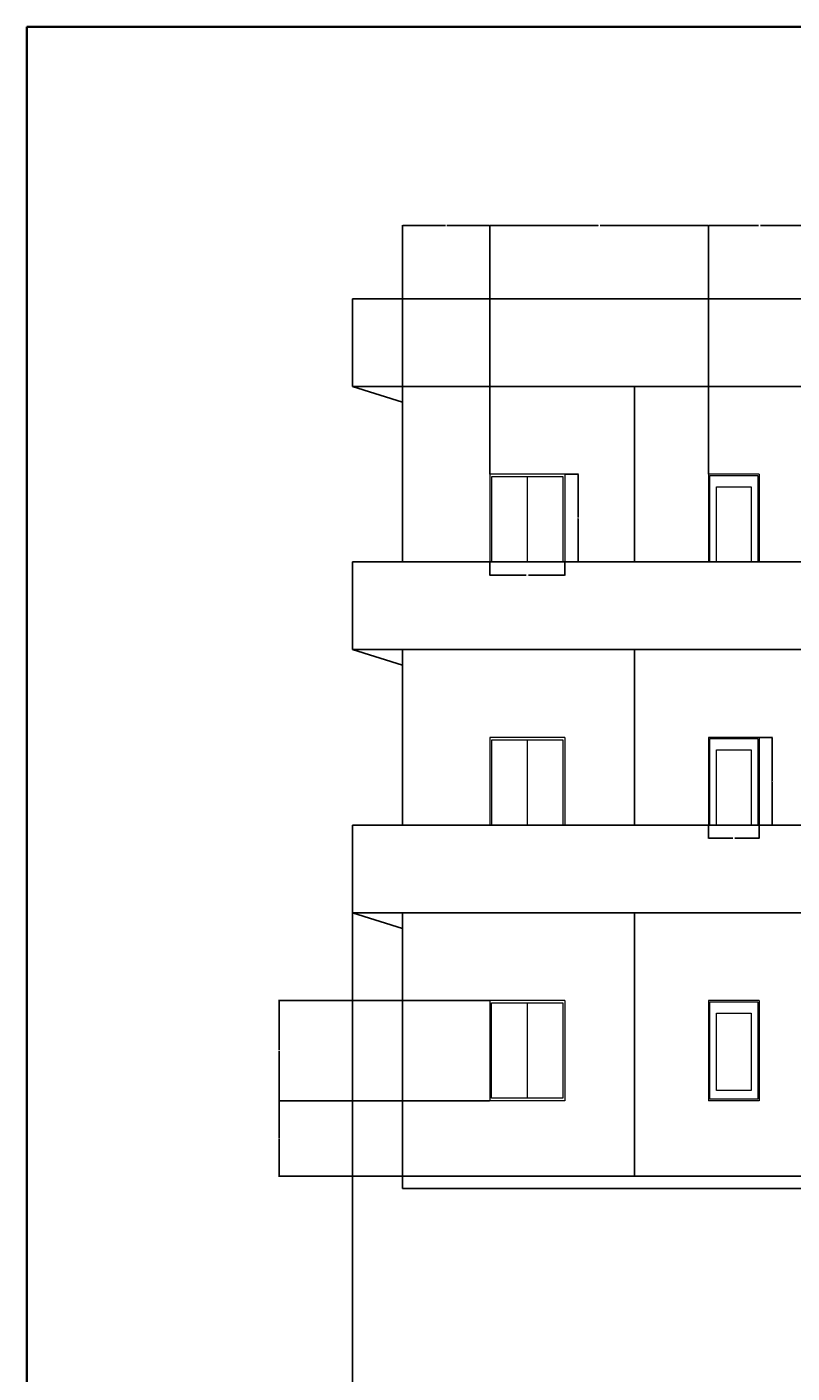
# Model space of a CAD drawing. Units: inches. Extents: x 1520 to 3401, y 1570 to 3432.
# Tile 8 of 15: x 1520 to 1886, y 2787 to 3432. Entities that reach past the tile are written whole.
import ezdxf

# ---------------------------------------------------------------- set-up
doc = ezdxf.new("R2010")
doc.units = ezdxf.units.IN
for name, color, linetype, lineweight in [('A-ANNO-DIMS', 2, 'Continuous', 18), ('A-ANNO-TTLB', 7, 'Continuous', 35), ('A-ELEV', 7, 'Continuous', 25), ('A-ELEV-GLAZ', 4, 'Continuous', 18)]:
    doc.layers.add(name, color=color, linetype=linetype, lineweight=lineweight)
doc.styles.get("Standard").update_dxf_attribs({"font": 'arial.ttf'})
doc.dimstyles.get("Standard").update_dxf_attribs({"dimtxt": 0.18, "dimasz": 0.18, "dimexe": 0.18, "dimexo": 0.0625, "dimgap": 0.09, "dimtad": 0, "dimtih": 1, "dimtoh": 1, "dimdec": 4, "dimzin": 0, "dimdsep": 46, "dimtxsty": 'Standard', "dimcen": 0.09, "dimadec": 0, "dimazin": 0, "dimtfac": 1, "dimtdec": 4, "dimtofl": 0, "dimtmove": 0, "dimatfit": 3, "dimfxl": 1, "dimtolj": 1, "dimtzin": 0, "dimarcsym": 0})

# ---------------------------------------------------------------- blocks, each defined once
blk = doc.blocks.new('WIN-ELEV-01')
for p, q in [((0, 42), (0, 0)), ((36, 42), (0, 42)), ((0, 42), (0, 0)), ((36, 42), (0, 42)), ((17.97, 40.89), (17.97, 0)), ((36, 42), (36, 0)), ((36, 42), (36, 0))]:
    blk.add_line(p, q)
blk.add_lwpolyline([(0.93, 0), (0.93, 40.89), (35, 40.89), (35, 0)])
blk = doc.blocks.new('WIN-ELEV-02')
for p, q in [((0, 42), (0, 0)), ((24.17, 42), (0, 42)), ((0, 42), (0, 0)), ((24.17, 42), (0, 42)), ((24.17, 42), (24.17, 0)), ((24.17, 42), (24.17, 0))]:
    blk.add_line(p, q)
for points in [[(0.65, 0), (0.65, 41.38), (23.63, 41.38), (23.63, 0)], [(3.78, 0), (3.78, 35.97), (20.43, 35.97), (20.43, 0)]]:
    blk.add_lwpolyline(points)
blk = doc.blocks.new('*D157')
at = {"layer": 'A-ANNO-DIMS', "color": 0, "lineweight": -2, "transparency": 16777216}
for p, q in [((1777.36, 3217.63), (1783.78, 3217.63)), ((1783.6, 3217.45), (1783.6, 3196.81)), ((1783.6, 3175.81), (1783.6, 3196.45)), ((1777.36, 3175.63), (1783.78, 3175.63))]:
    blk.add_line(p, q, dxfattribs=at)
at = {"layer": 'A-ANNO-DIMS', "color": 0, "transparency": 16777216}
for points in [[(1783.57, 3217.45), (1783.63, 3217.45), (1783.6, 3217.63)], [(1783.57, 3175.81), (1783.63, 3175.81), (1783.6, 3175.63)]]:
    blk.add_solid(points, dxfattribs=at)
at = {"layer": 'Defpoints', "color": 0, "transparency": 16777216}
for p in [(1777.3, 3217.63), (1783.6, 3217.63), (1777.3, 3175.63)]:
    blk.add_point(p, dxfattribs=at)
at = {"layer": 'A-ANNO-DIMS', "color": 0, "transparency": 16777216, "insert": (1783.6, 3196.63), "char_height": 0.18, "attachment_point": 5}
blk.add_mtext('\\A1;EW1 42 TYP.', dxfattribs=at)
blk = doc.blocks.new('*D158')
at = {"layer": 'A-ANNO-DIMS', "color": 0, "lineweight": -2, "transparency": 16777216}
for p, q in [((1741.3, 3175.57), (1741.3, 3169.15)), ((1777.3, 3175.57), (1777.3, 3169.15)), ((1741.48, 3169.33), (1758.77, 3169.33)), ((1777.12, 3169.33), (1759.82, 3169.33))]:
    blk.add_line(p, q, dxfattribs=at)
at = {"layer": 'A-ANNO-DIMS', "color": 0, "transparency": 16777216}
for points in [[(1741.48, 3169.36), (1741.48, 3169.3), (1741.3, 3169.33)], [(1777.12, 3169.36), (1777.12, 3169.3), (1777.3, 3169.33)]]:
    blk.add_solid(points, dxfattribs=at)
at = {"layer": 'Defpoints', "color": 0, "transparency": 16777216}
for p in [(1741.3, 3175.63), (1777.3, 3175.63), (1777.3, 3169.33)]:
    blk.add_point(p, dxfattribs=at)
at = {"layer": 'A-ANNO-DIMS', "color": 0, "transparency": 16777216, "insert": (1759.3, 3169.33), "char_height": 0.18, "attachment_point": 5}
blk.add_mtext('\\A1;36 TYP.', dxfattribs=at)
blk = doc.blocks.new('*D159')
at = {"layer": 'A-ANNO-DIMS', "color": 0, "lineweight": -2, "transparency": 16777216}
for p, q in [((1870.19, 3091.63), (1876.61, 3091.63)), ((1876.43, 3091.45), (1876.43, 3070.81)), ((1876.43, 3049.81), (1876.43, 3070.45)), ((1870.19, 3049.63), (1876.61, 3049.63))]:
    blk.add_line(p, q, dxfattribs=at)
at = {"layer": 'A-ANNO-DIMS', "color": 0, "transparency": 16777216}
for points in [[(1876.4, 3091.45), (1876.46, 3091.45), (1876.43, 3091.63)], [(1876.4, 3049.81), (1876.46, 3049.81), (1876.43, 3049.63)]]:
    blk.add_solid(points, dxfattribs=at)
at = {"layer": 'Defpoints', "color": 0, "transparency": 16777216}
for p in [(1870.13, 3091.63), (1876.43, 3091.63), (1870.13, 3049.63)]:
    blk.add_point(p, dxfattribs=at)
at = {"layer": 'A-ANNO-DIMS', "color": 0, "transparency": 16777216, "insert": (1876.43, 3070.63), "char_height": 0.18, "attachment_point": 5}
blk.add_mtext('\\A1;EW2 42 TYP.', dxfattribs=at)
blk = doc.blocks.new('*D160')
at = {"layer": 'A-ANNO-DIMS', "color": 0, "lineweight": -2, "transparency": 16777216}
for p, q in [((1845.96, 3049.57), (1845.96, 3043.15)), ((1870.13, 3049.57), (1870.13, 3043.15)), ((1846.14, 3043.33), (1857.51, 3043.33)), ((1869.95, 3043.33), (1858.57, 3043.33))]:
    blk.add_line(p, q, dxfattribs=at)
at = {"layer": 'A-ANNO-DIMS', "color": 0, "transparency": 16777216}
for points in [[(1846.14, 3043.36), (1846.14, 3043.3), (1845.96, 3043.33)], [(1869.95, 3043.36), (1869.95, 3043.3), (1870.13, 3043.33)]]:
    blk.add_solid(points, dxfattribs=at)
at = {"layer": 'Defpoints', "color": 0, "transparency": 16777216}
for p in [(1845.96, 3049.63), (1870.13, 3049.63), (1870.13, 3043.33)]:
    blk.add_point(p, dxfattribs=at)
at = {"layer": 'A-ANNO-DIMS', "color": 0, "transparency": 16777216, "insert": (1858.04, 3043.33), "char_height": 0.18, "attachment_point": 5}
blk.add_mtext('\\A1;24 TYP.', dxfattribs=at)
blk = doc.blocks.new('*D209')
at = {"layer": 'A-ANNO-DIMS', "color": 0, "lineweight": -2, "transparency": 16777216}
for p, q in [((1675.61, 3007.57), (1675.61, 2752.86)), ((2368.11, 3007.57), (2368.11, 2752.86)), ((1675.79, 2753.04), (2021.47, 2753.04)), ((2367.93, 2753.04), (2022.26, 2753.04))]:
    blk.add_line(p, q, dxfattribs=at)
at = {"layer": 'A-ANNO-DIMS', "color": 0, "transparency": 16777216}
for points in [[(1675.79, 2753.07), (1675.79, 2753.01), (1675.61, 2753.04)], [(2367.93, 2753.07), (2367.93, 2753.01), (2368.11, 2753.04)]]:
    blk.add_solid(points, dxfattribs=at)
at = {"layer": 'Defpoints', "color": 0, "transparency": 16777216}
for p in [(1675.61, 3007.63), (2368.11, 3007.63), (2368.11, 2753.04)]:
    blk.add_point(p, dxfattribs=at)
at = {"layer": 'A-ANNO-DIMS', "color": 0, "transparency": 16777216, "insert": (2021.86, 2753.04), "char_height": 0.18, "attachment_point": 5}
blk.add_mtext('\\A1;692.5', dxfattribs=at)
blk = doc.blocks.new('*D212')
at = {"layer": 'A-ANNO-DIMS', "color": 0, "lineweight": -2, "transparency": 16777216}
for p, q in [((1741.23, 2917.63), (1640.33, 2917.63)), ((1640.51, 2917.45), (1640.51, 2899.81)), ((1640.51, 2881.81), (1640.51, 2899.45)), ((1699.55, 2881.63), (1640.33, 2881.63))]:
    blk.add_line(p, q, dxfattribs=at)
at = {"layer": 'A-ANNO-DIMS', "color": 0, "transparency": 16777216}
for points in [[(1640.48, 2917.45), (1640.54, 2917.45), (1640.51, 2917.63)], [(1640.48, 2881.81), (1640.54, 2881.81), (1640.51, 2881.63)]]:
    blk.add_solid(points, dxfattribs=at)
at = {"layer": 'Defpoints', "color": 0, "transparency": 16777216}
for p in [(1640.51, 2917.63), (1741.3, 2917.63), (1699.61, 2881.63)]:
    blk.add_point(p, dxfattribs=at)
at = {"layer": 'A-ANNO-DIMS', "color": 0, "transparency": 16777216, "insert": (1640.51, 2899.63), "char_height": 0.18, "attachment_point": 5}
blk.add_mtext('\\A1;36', dxfattribs=at)
blk = doc.blocks.new('*D213')
at = {"layer": 'A-ANNO-DIMS', "color": 0, "lineweight": -2, "transparency": 16777216}
for p, q in [((1741.23, 2965.63), (1640.33, 2965.63)), ((1640.51, 2965.45), (1640.51, 2941.81)), ((1640.51, 2917.81), (1640.51, 2941.45)), ((1741.23, 2917.63), (1640.33, 2917.63))]:
    blk.add_line(p, q, dxfattribs=at)
at = {"layer": 'A-ANNO-DIMS', "color": 0, "transparency": 16777216}
for points in [[(1640.48, 2965.45), (1640.54, 2965.45), (1640.51, 2965.63)], [(1640.48, 2917.81), (1640.54, 2917.81), (1640.51, 2917.63)]]:
    blk.add_solid(points, dxfattribs=at)
at = {"layer": 'Defpoints', "color": 0, "transparency": 16777216}
for p in [(1640.51, 2965.63), (1741.3, 2965.63), (1741.3, 2917.63)]:
    blk.add_point(p, dxfattribs=at)
at = {"layer": 'A-ANNO-DIMS', "color": 0, "transparency": 16777216, "insert": (1640.51, 2941.63), "char_height": 0.18, "attachment_point": 5}
blk.add_mtext('\\A1;48', dxfattribs=at)
blk = doc.blocks.new('*D215')
at = {"layer": 'A-ANNO-DIMS', "color": 0, "lineweight": -2, "transparency": 16777216}
for p, q in [((1699.61, 3259.7), (1699.61, 3336.91)), ((1699.79, 3336.73), (1720.06, 3336.73)), ((1741.12, 3336.73), (1720.85, 3336.73)), ((1741.3, 3217.7), (1741.3, 3336.91))]:
    blk.add_line(p, q, dxfattribs=at)
at = {"layer": 'A-ANNO-DIMS', "color": 0, "transparency": 16777216}
for points in [[(1699.79, 3336.76), (1699.79, 3336.7), (1699.61, 3336.73)], [(1741.12, 3336.76), (1741.12, 3336.7), (1741.3, 3336.73)]]:
    blk.add_solid(points, dxfattribs=at)
at = {"layer": 'Defpoints', "color": 0, "transparency": 16777216}
for p in [(1741.3, 3336.73), (1699.61, 3259.63), (1741.3, 3217.63)]:
    blk.add_point(p, dxfattribs=at)
at = {"layer": 'A-ANNO-DIMS', "color": 0, "transparency": 16777216, "insert": (1720.45, 3336.73), "char_height": 0.18, "attachment_point": 5}
blk.add_mtext('\\A1;41.68', dxfattribs=at)
blk = doc.blocks.new('*D216')
at = {"layer": 'A-ANNO-DIMS', "color": 0, "lineweight": -2, "transparency": 16777216}
for p, q in [((1741.3, 3217.7), (1741.3, 3336.91)), ((1741.48, 3336.73), (1793.17, 3336.73)), ((1845.78, 3336.73), (1794.08, 3336.73)), ((1845.96, 3217.7), (1845.96, 3336.91))]:
    blk.add_line(p, q, dxfattribs=at)
at = {"layer": 'A-ANNO-DIMS', "color": 0, "transparency": 16777216}
for points in [[(1741.48, 3336.76), (1741.48, 3336.7), (1741.3, 3336.73)], [(1845.78, 3336.76), (1845.78, 3336.7), (1845.96, 3336.73)]]:
    blk.add_solid(points, dxfattribs=at)
at = {"layer": 'Defpoints', "color": 0, "transparency": 16777216}
for p in [(1845.96, 3336.73), (1741.3, 3217.63), (1845.96, 3217.63)]:
    blk.add_point(p, dxfattribs=at)
at = {"layer": 'A-ANNO-DIMS', "color": 0, "transparency": 16777216, "insert": (1793.63, 3336.73), "char_height": 0.18, "attachment_point": 5}
blk.add_mtext('\\A1;104.66', dxfattribs=at)
blk = doc.blocks.new('*D217')
at = {"layer": 'A-ANNO-DIMS', "color": 0, "lineweight": -2, "transparency": 16777216}
for p, q in [((1845.96, 3217.7), (1845.96, 3336.91)), ((1846.14, 3336.73), (1869.94, 3336.73)), ((1894.55, 3336.73), (1870.74, 3336.73)), ((1894.73, 3217.7), (1894.73, 3336.91))]:
    blk.add_line(p, q, dxfattribs=at)
at = {"layer": 'A-ANNO-DIMS', "color": 0, "transparency": 16777216}
for points in [[(1846.14, 3336.76), (1846.14, 3336.7), (1845.96, 3336.73)], [(1894.55, 3336.76), (1894.55, 3336.7), (1894.73, 3336.73)]]:
    blk.add_solid(points, dxfattribs=at)
at = {"layer": 'Defpoints', "color": 0, "transparency": 16777216}
for p in [(1894.73, 3336.73), (1845.96, 3217.63), (1894.73, 3217.63)]:
    blk.add_point(p, dxfattribs=at)
at = {"layer": 'A-ANNO-DIMS', "color": 0, "transparency": 16777216, "insert": (1870.34, 3336.73), "char_height": 0.18, "attachment_point": 5}
blk.add_mtext('\\A1;48.77', dxfattribs=at)

msp = doc.modelspace()

# ---------------------------------------------------------------- linework, layer by layer
at = {"layer": 'A-ANNO-TTLB'}
msp.add_lwpolyline([(1519.9253, 3431.7421), (3400.8761, 3431.7421), (3400.8761, 1570.3458), (1519.9253, 1570.3458)], close=True, dxfattribs=at)
at = {"layer": 'A-ELEV'}
for p, q in [((2368.1128, 3301.633), (1675.6128, 3301.633)), ((1675.6128, 3259.633), (1675.6128, 3301.633)), ((2368.1128, 3259.633), (1675.6128, 3259.633)), ((1675.6128, 3259.633), (1699.6128, 3252.133)), ((1699.6128, 3259.633), (1699.6128, 3175.633)), ((1810.5002, 3175.633), (1810.5002, 3259.633)), ((2368.1128, 3175.633), (1675.6128, 3175.633)), ((1675.6128, 3133.633), (1675.6128, 3175.633)), ((2368.1128, 3133.633), (1675.6128, 3133.633)), ((1675.6128, 3133.633), (1699.6128, 3126.133)), ((1699.6128, 3133.633), (1699.6128, 3049.633)), ((1699.6128, 3133.633), (1699.6128, 3118.633)), ((1810.5002, 3049.633), (1810.5002, 3133.633)), ((2368.1128, 3049.633), (1675.6128, 3049.633)), ((1675.6128, 3007.633), (1675.6128, 3049.633)), ((2368.1128, 3007.633), (1675.6128, 3007.633)), ((1675.6128, 3007.633), (1699.6128, 3000.133)), ((1699.6128, 3007.633), (1699.6128, 2875.633)), ((1699.6128, 3007.633), (1699.6128, 2992.633)), ((1810.5002, 2881.633), (1810.5002, 3007.633)), ((2344.1128, 2881.633), (1699.6128, 2881.633)), ((1699.6128, 2881.633), (1699.6128, 2875.633)), ((1699.6128, 2875.633), (2344.1128, 2875.633))]:
    msp.add_line(p, q, dxfattribs=at)
at = {"layer": 'A-ELEV-GLAZ'}
for p, q in [((1741.2966, 2965.633), (1741.2966, 2917.633)), ((1777.2966, 2965.633), (1741.2966, 2965.633)), ((1759.2622, 2964.5201), (1759.2622, 2918.979)), ((1777.2966, 2965.633), (1777.2966, 2917.633)), ((1845.9552, 2965.633), (1845.9552, 2917.633)), ((1870.1255, 2965.633), (1845.9552, 2965.633)), ((1870.1255, 2965.633), (1870.1255, 2917.633)), ((1777.2966, 2917.633), (1741.2966, 2917.633)), ((1870.1255, 2917.633), (1845.9552, 2917.633))]:
    msp.add_line(p, q, dxfattribs=at)
for points in [[(1742.2228, 2964.5201), (1776.3017, 2964.5201), (1776.3017, 2918.979), (1742.2228, 2918.979)], [(1846.6068, 2965.0099), (1869.5875, 2965.0099), (1869.5875, 2918.4582), (1846.6068, 2918.4582)], [(1849.7367, 2959.5992), (1866.3874, 2959.5992), (1866.3874, 2922.5918), (1849.7367, 2922.5918)]]:
    msp.add_lwpolyline(points, close=True, dxfattribs=at)

# ---------------------------------------------------------------- block references
for name, p in [('WIN-ELEV-01', (1741.297, 3175.633)), ('WIN-ELEV-02', (1845.955, 3175.633)), ('WIN-ELEV-01', (1741.297, 3049.633)), ('WIN-ELEV-02', (1845.955, 3049.633))]:
    msp.add_blockref(name, p, dxfattribs=at)

# ---------------------------------------------------------------- dimensions: what is measured, and where the dimension line sits
at = {"layer": 'A-ANNO-DIMS'}
for base, p1, p2, override, picture, middle in [((1741.2966, 3336.733), (1699.6128, 3259.633), (1741.2966, 3217.633), {"dimdec": 2, "dimlfac": 1, "dimrnd": 0, "dimzin": 0, "dimdsep": 46, "dimlunit": 2}, '*D215', (1720.4547, 3336.733)), ((1845.9552, 3336.733), (1741.2966, 3217.633), (1845.9552, 3217.633), {"dimdec": 2, "dimlfac": 1, "dimrnd": 0, "dimzin": 0, "dimdsep": 46, "dimlunit": 2}, '*D216', (1793.6259, 3336.733)), ((1894.7277, 3336.733), (1845.9552, 3217.633), (1894.7277, 3217.633), {"dimdec": 2, "dimlfac": 1, "dimrnd": 0, "dimzin": 0, "dimdsep": 46, "dimlunit": 2}, '*D217', (1870.3415, 3336.733)), ((2368.1128, 2753.0384), (1675.6128, 3007.633), (2368.1128, 3007.633), {"dimdec": 1, "dimlfac": 1, "dimrnd": 0, "dimzin": 0, "dimdsep": 46, "dimlunit": 2}, '*D209', (2021.8628, 2753.0384))]:
    dim = msp.add_linear_dim(base=base, p1=p1, p2=p2, dimstyle='Standard', override=override, dxfattribs=at)
    dim.commit()
    dim.dimension.update_dxf_attribs({"geometry": picture, "text_midpoint": middle})
for base, p1, p2, text, picture, middle in [((1783.5966, 3217.633), (1777.2966, 3175.633), (1777.2966, 3217.633), 'EW1 <> TYP.', '*D157', (1783.5966, 3196.633)), ((1876.4255, 3091.633), (1870.1255, 3049.633), (1870.1255, 3091.633), 'EW2 <> TYP.', '*D159', (1876.4255, 3070.633))]:
    dim = msp.add_linear_dim(base=base, p1=p1, p2=p2, angle=90, text=text, dimstyle='Standard', override={"dimdec": 0, "dimlfac": 1, "dimrnd": 0, "dimzin": 0, "dimdsep": 46, "dimlunit": 2}, dxfattribs=at)
    dim.commit()
    dim.dimension.update_dxf_attribs({"geometry": picture, "text_midpoint": middle})
for base, p1, p2, picture, middle in [((1777.2966, 3169.333), (1741.2966, 3175.633), (1777.2966, 3175.633), '*D158', (1759.2966, 3169.333)), ((1870.1255, 3043.333), (1845.9552, 3049.633), (1870.1255, 3049.633), '*D160', (1858.0404, 3043.333))]:
    dim = msp.add_linear_dim(base=base, p1=p1, p2=p2, text='<> TYP.', dimstyle='Standard', override={"dimdec": 0, "dimlfac": 1, "dimrnd": 0, "dimzin": 0, "dimdsep": 46, "dimlunit": 2}, dxfattribs=at)
    dim.commit()
    dim.dimension.update_dxf_attribs({"geometry": picture, "text_midpoint": middle})
for base, p1, p2, picture, middle in [((1640.5128, 2965.633), (1741.2966, 2917.633), (1741.2966, 2965.633), '*D213', (1640.5128, 2941.633)), ((1640.5128, 2917.633), (1699.6128, 2881.633), (1741.2966, 2917.633), '*D212', (1640.5128, 2899.633))]:
    dim = msp.add_linear_dim(base=base, p1=p1, p2=p2, angle=90, dimstyle='Standard', override={"dimdec": 0, "dimlfac": 1, "dimrnd": 0, "dimzin": 0, "dimdsep": 46, "dimlunit": 2}, dxfattribs=at)
    dim.commit()
    dim.dimension.update_dxf_attribs({"geometry": picture, "text_midpoint": middle})

doc.saveas('drawing.dxf')
